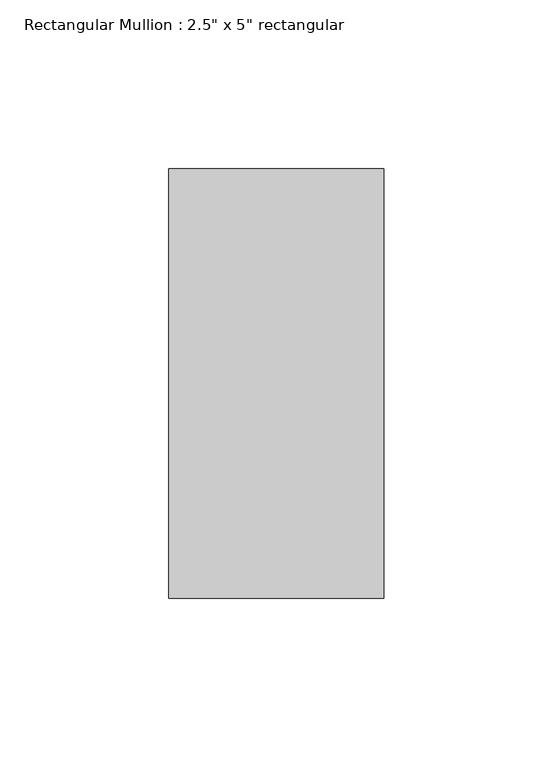
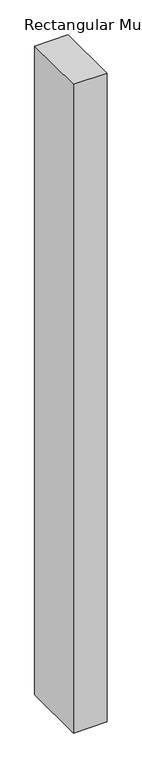
"""IFC4 building model written with IfcOpenShell, lengths in millimetres: member geometry."""

from ifc_helpers import new_model, si_unit, frame, origin, place, context, project, spatial, polyline, outline, extrude, source, transform, mapped, element, save


def member_a88312ef(model_context):
    return source(origin(), model_context, "Body", "SweptSolid", [
        extrude(outline(polyline([(31.75, 63.5), (31.75, -63.5), (-31.75, -63.5), (-31.75, 63.5), (31.75, 63.5)])), frame((0.0, 0.0, -1298.2581531), z_axis=(0.0, 0.0, 1.0), x_axis=(1.0, 0.0, 0.0)), (0.0, 0.0, 1.0), 1298.2581531),
    ])


if __name__ == "__main__":
    model = new_model("IFC4")
    model_context = context("Model", 3, world=origin())
    ifc_project = project(units=[si_unit("LENGTHUNIT", "METRE", prefix="MILLI")], contexts=[model_context])
    site = spatial("IfcSite", under=ifc_project)
    building = spatial("IfcBuilding", under=site)
    placement = place(None, origin())
    member_shape = member_a88312ef(model_context)
    element("IfcMember", 1, ObjectType="Rectangular Mullion : 2.5\" x 5\" rectangular", at=placement, inside=building, context=model_context, shape_type="MappedRepresentation", body=[
        mapped(member_shape, transform((0.0, 0.0, 0.0), x_axis=(1.0, 0.0, 0.0), y_axis=(0.0, 1.0, 0.0), z_axis=(0.0, 0.0, 1.0))),
    ])
    save(model, "model.ifc")

# Revit data of these elements
# Type "Rectangular Mullion : 2.5\" x 5\" rectangular"
#   built-in parameter 1007304 = 0.416667 (stored number, unit not read)
#   built-in parameter 1007301 = 0.104167 (stored number, unit not read)
#   built-in parameter 1007300 = 0.104167 (stored number, unit not read)
# Element 1 (IfcMember, "Rectangular Mullion : 2.5\" x 5\" rectangular")
#   Materials on its faces: "Aluminum"
# Materials
#   "Aluminum": class "Metal", colour RGB 247 247 247, transparency 0, Description = "Aluminum 6061", Cost = 0
